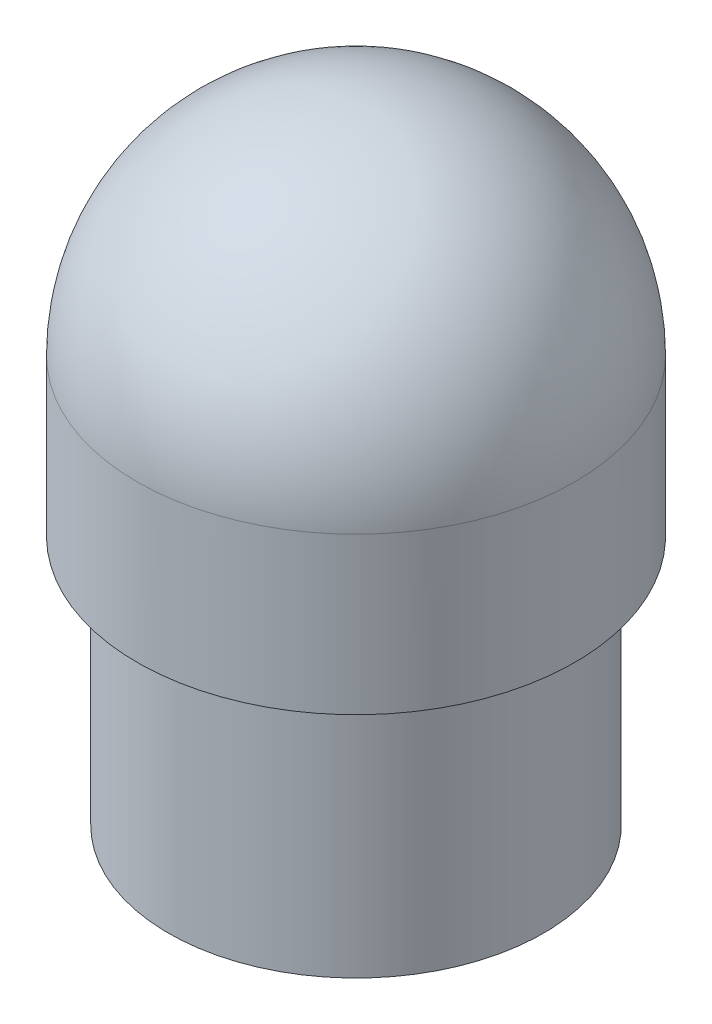
from build123d import *


with BuildPart() as part:
    # Pin Profile Sketch → Pin Body Revolve (revolve)
    with BuildSketch(Plane.XY, mode=Mode.PRIVATE) as pin_body_revolve_sk:
        with BuildLine():
            Line((0, 0), (15, 0))
            Line((15, 0), (15, 20))
            Line((15, 20), (17.5, 20))
            Line((17.5, 20), (17.5, 32.5))
            ThreePointArc((17.5, 32.5), (12.374368671, 44.874368671), (0, 50))
            Line((0, 50), (0, 0))
        make_face()
    revolve(pin_body_revolve_sk.sketch.rotate(Axis((0, 50, 0), (0, -1, 0)), 180), axis=Axis((0, 50, 0), (0, -1, 0)))


solid = part.part
